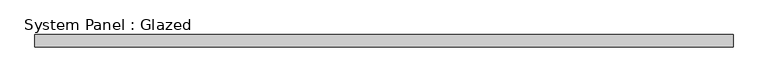
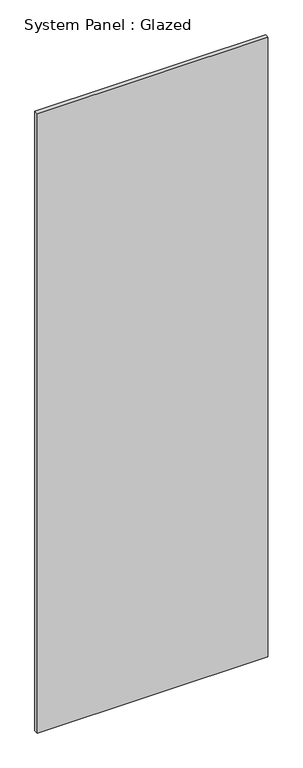
"""IFC4 building model written with IfcOpenShell, lengths in millimetres: plate geometry, System Panel : Glazed."""

from ifc_helpers import new_model, si_unit, origin, origin_with_axes, place, context, project, spatial, polyline, outline, extrude, source, transform, mapped, element, save


def system_panel_glazed_dc9dfaf4(model_context):
    return source(origin(), model_context, "Body", "SweptSolid", [
        extrude(outline(polyline([(729.1088716, 19.05), (-729.1088716, 19.05), (-729.1088716, 44.45), (729.1088716, 44.45), (729.1088716, 19.05)])), origin_with_axes(), (0.0, 0.0, 1.0), 4140.2),
    ])


if __name__ == "__main__":
    model = new_model("IFC4")
    model_context = context("Model", 3, world=origin())
    ifc_project = project(units=[si_unit("LENGTHUNIT", "METRE", prefix="MILLI")], contexts=[model_context])
    site = spatial("IfcSite", under=ifc_project)
    building = spatial("IfcBuilding", under=site)
    placement = place(None, origin())
    system_panel_glazed_shape = system_panel_glazed_dc9dfaf4(model_context)
    element("IfcPlate", 1, ObjectType="System Panel : Glazed", at=placement, inside=building, context=model_context, shape_type="MappedRepresentation", body=[
        mapped(system_panel_glazed_shape, transform((0.0, 0.0, 0.0), x_axis=(1.0, 0.0, 0.0), y_axis=(0.0, 1.0, 0.0), z_axis=(0.0, 0.0, 1.0))),
    ])
    save(model, "model.ifc")

# Revit data of these elements
# Type "System Panel : Glazed"
#   Construction Type Id = "GSP4R"
#   Analytic Construction = "1/8 in Pilkington single glazing"
#   Visual Light Transmittance = 0.9
#   Solar Heat Gain Coefficient = 0.86
#   Heat Transfer Coefficient (U) = 1.18115 BTU/(h·ft²·°F)
# Element 1 (IfcPlate, "System Panel : Glazed")
#   Materials on its faces: "Glass"
# Materials
#   "Glass": class "Glass", colour RGB 0 128 192, transparency 0.75, Description = "Soda Lime Glass", Cost = 0
